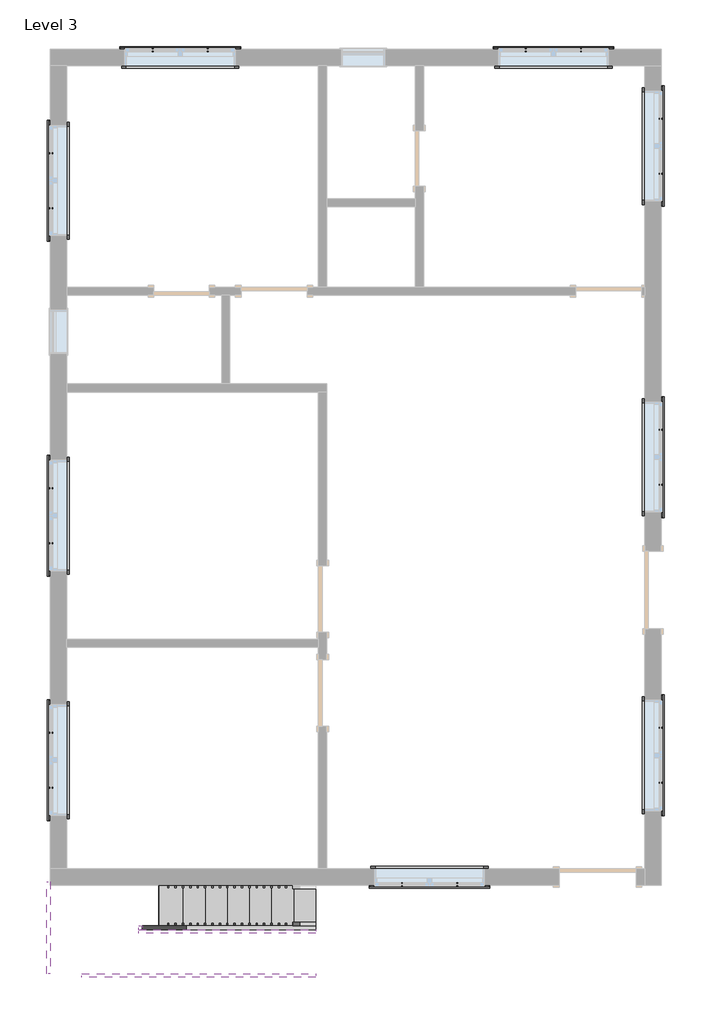
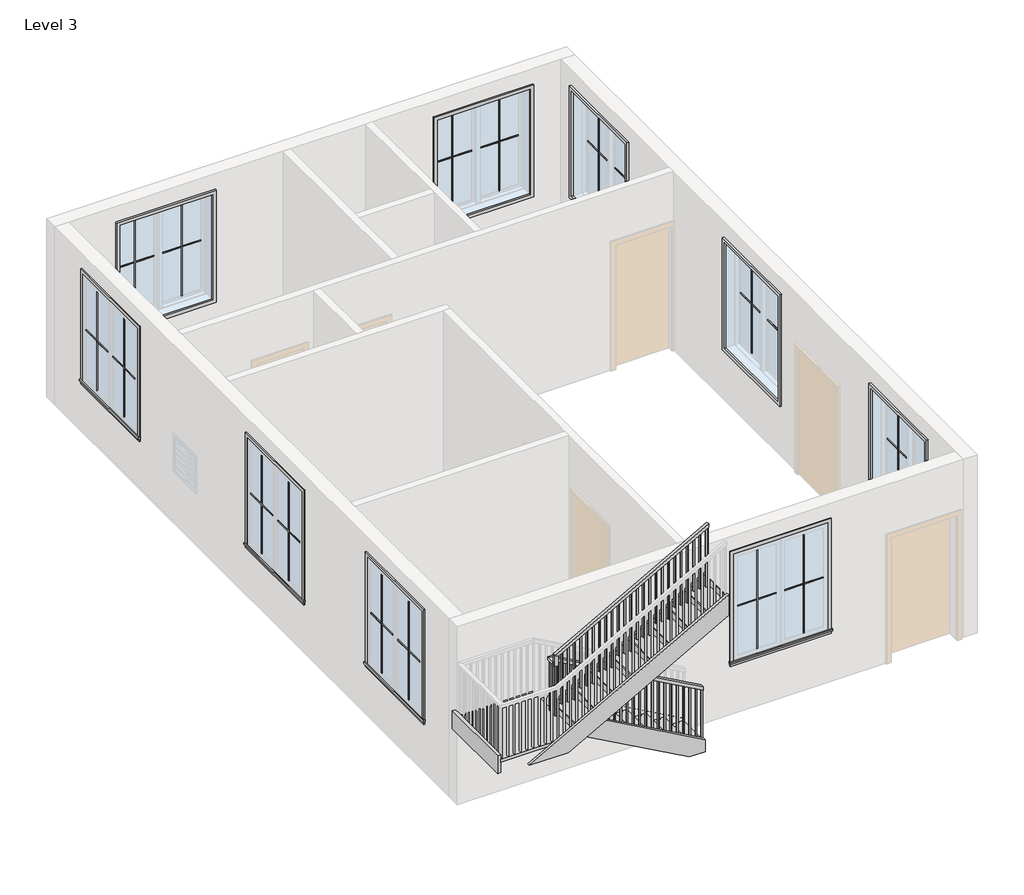
# One storey, part 3 of 3: 36 proxies, 6 members, 1 railing, 1 stair flight.
"""IFC4 building model written with IfcOpenShell, lengths in millimetres."""

from ifc_helpers import new_model, si_unit, frame, origin, place, context, project, spatial, polyline, outline, extrude, faceted_brep, transform, mapped, element, save
from components import muntin_pattern_2x2_muntin_pattern_2x2_f6a80940, muntin_pattern_2x2_muntin_pattern_2x2_09b00a1c, trim_window_exterior_flat_with_sill_698ed857, trim_window_interior_flat_picture_frame_92551a5e, stair_flight_17867b1e

model = new_model("IFC4")

# Units and contexts
model_context = context("Model", 3, world=origin())
ifc_project = project(units=[si_unit("LENGTHUNIT", "METRE", prefix="MILLI")], contexts=[model_context])

# Site, building, storey
site = spatial("IfcSite", under=ifc_project)
building = spatial("IfcBuilding", under=site)
storey = spatial("IfcBuildingStorey", under=building, Name="Level 3", Elevation=3200.4)

# Proxies
placement = place(None, origin())
muntin_pattern_2x2_muntin_pattern_2x2_shape = muntin_pattern_2x2_muntin_pattern_2x2_f6a80940(model_context)
element("IfcBuildingElementProxy", 1, Name="Muntin Pattern_2x2 : Muntin Pattern_2x2", ObjectType="Muntin Pattern_2x2 : Muntin Pattern_2x2", at=placement, inside=storey, context=model_context, shape_type="MappedRepresentation", body=[
    mapped(muntin_pattern_2x2_muntin_pattern_2x2_shape, transform((-5453.9948569, -3961.7808037, 4184.65), x_axis=(0.0, 1.0, 0.0), y_axis=(-1.0, 0.0, 0.0), z_axis=(0.0, 0.0, 1.0))),
])
element("IfcBuildingElementProxy", 2, Name="Muntin Pattern_2x2 : Muntin Pattern_2x2", ObjectType="Muntin Pattern_2x2 : Muntin Pattern_2x2", at=placement, inside=storey, context=model_context, shape_type="MappedRepresentation", body=[
    mapped(muntin_pattern_2x2_muntin_pattern_2x2_shape, transform((-5453.9948569, -593.1058037, 4184.65), x_axis=(0.0, 1.0, 0.0), y_axis=(-1.0, 0.0, 0.0), z_axis=(0.0, 0.0, 1.0))),
])
element("IfcBuildingElementProxy", 3, Name="Muntin Pattern_2x2 : Muntin Pattern_2x2", ObjectType="Muntin Pattern_2x2 : Muntin Pattern_2x2", at=placement, inside=storey, context=model_context, shape_type="MappedRepresentation", body=[
    mapped(muntin_pattern_2x2_muntin_pattern_2x2_shape, transform((-5453.9948569, 4023.3441963, 4184.65), x_axis=(0.0, 1.0, 0.0), y_axis=(-1.0, 0.0, 0.0), z_axis=(0.0, 0.0, 1.0))),
])
element("IfcBuildingElementProxy", 4, Name="Muntin Pattern_2x2 : Muntin Pattern_2x2", ObjectType="Muntin Pattern_2x2 : Muntin Pattern_2x2", at=placement, inside=storey, context=model_context, shape_type="MappedRepresentation", body=[
    mapped(muntin_pattern_2x2_muntin_pattern_2x2_shape, transform((2947.0551431, 5258.4191963, 4184.65), x_axis=(0.0, -1.0, 0.0), y_axis=(1.0, 0.0, 0.0), z_axis=(0.0, 0.0, 1.0))),
])
element("IfcBuildingElementProxy", 5, Name="Muntin Pattern_2x2 : Muntin Pattern_2x2", ObjectType="Muntin Pattern_2x2 : Muntin Pattern_2x2", at=placement, inside=storey, context=model_context, shape_type="MappedRepresentation", body=[
    mapped(muntin_pattern_2x2_muntin_pattern_2x2_shape, transform((2947.0551431, 972.1691963, 4184.65), x_axis=(0.0, -1.0, 0.0), y_axis=(1.0, 0.0, 0.0), z_axis=(0.0, 0.0, 1.0))),
])
element("IfcBuildingElementProxy", 6, Name="Muntin Pattern_2x2 : Muntin Pattern_2x2", ObjectType="Muntin Pattern_2x2 : Muntin Pattern_2x2", at=placement, inside=storey, context=model_context, shape_type="MappedRepresentation", body=[
    mapped(muntin_pattern_2x2_muntin_pattern_2x2_shape, transform((2947.0551431, -3136.2808037, 4184.65), x_axis=(0.0, -1.0, 0.0), y_axis=(1.0, 0.0, 0.0), z_axis=(0.0, 0.0, 1.0))),
])
element("IfcBuildingElementProxy", 7, Name="Muntin Pattern_2x2 : Muntin Pattern_2x2", ObjectType="Muntin Pattern_2x2 : Muntin Pattern_2x2", at=placement, inside=storey, context=model_context, shape_type="MappedRepresentation", body=[
    mapped(muntin_pattern_2x2_muntin_pattern_2x2_shape, transform((141.9426431, -5296.8683037, 4184.65), x_axis=(-1.0, 0.0, 0.0), y_axis=(0.0, -1.0, 0.0), z_axis=(0.0, 0.0, 1.0))),
])
element("IfcBuildingElementProxy", 8, Name="Muntin Pattern_2x2 : Muntin Pattern_2x2", ObjectType="Muntin Pattern_2x2 : Muntin Pattern_2x2", at=placement, inside=storey, context=model_context, shape_type="MappedRepresentation", body=[
    mapped(muntin_pattern_2x2_muntin_pattern_2x2_shape, transform((1091.2676431, 6202.9816963, 4184.65), x_axis=(1.0, 0.0, 0.0), y_axis=(0.0, 1.0, 0.0), z_axis=(0.0, 0.0, 1.0))),
])
element("IfcBuildingElementProxy", 9, Name="Muntin Pattern_2x2 : Muntin Pattern_2x2", ObjectType="Muntin Pattern_2x2 : Muntin Pattern_2x2", at=placement, inside=storey, context=model_context, shape_type="MappedRepresentation", body=[
    mapped(muntin_pattern_2x2_muntin_pattern_2x2_shape, transform((-4052.2323569, 6202.9816963, 4184.65), x_axis=(1.0, 0.0, 0.0), y_axis=(0.0, 1.0, 0.0), z_axis=(0.0, 0.0, 1.0))),
])
muntin_pattern_2x2_muntin_pattern_2x2_2_shape = muntin_pattern_2x2_muntin_pattern_2x2_09b00a1c(model_context)
element("IfcBuildingElementProxy", 10, Name="Muntin Pattern_2x2 : Muntin Pattern_2x2", ObjectType="Muntin Pattern_2x2 : Muntin Pattern_2x2", at=placement, inside=storey, context=model_context, shape_type="MappedRepresentation", body=[
    mapped(muntin_pattern_2x2_muntin_pattern_2x2_2_shape, transform((-5453.9948569, -3202.9558037, 4184.65), x_axis=(0.0, -1.0, 0.0), y_axis=(1.0, 0.0, 0.0), z_axis=(0.0, 0.0, 1.0))),
])
element("IfcBuildingElementProxy", 11, Name="Muntin Pattern_2x2 : Muntin Pattern_2x2", ObjectType="Muntin Pattern_2x2 : Muntin Pattern_2x2", at=placement, inside=storey, context=model_context, shape_type="MappedRepresentation", body=[
    mapped(muntin_pattern_2x2_muntin_pattern_2x2_2_shape, transform((-5453.9948569, 165.7191963, 4184.65), x_axis=(0.0, -1.0, 0.0), y_axis=(1.0, 0.0, 0.0), z_axis=(0.0, 0.0, 1.0))),
])
element("IfcBuildingElementProxy", 12, Name="Muntin Pattern_2x2 : Muntin Pattern_2x2", ObjectType="Muntin Pattern_2x2 : Muntin Pattern_2x2", at=placement, inside=storey, context=model_context, shape_type="MappedRepresentation", body=[
    mapped(muntin_pattern_2x2_muntin_pattern_2x2_2_shape, transform((-5453.9948569, 4782.1691963, 4184.65), x_axis=(0.0, -1.0, 0.0), y_axis=(1.0, 0.0, 0.0), z_axis=(0.0, 0.0, 1.0))),
])
element("IfcBuildingElementProxy", 13, Name="Muntin Pattern_2x2 : Muntin Pattern_2x2", ObjectType="Muntin Pattern_2x2 : Muntin Pattern_2x2", at=placement, inside=storey, context=model_context, shape_type="MappedRepresentation", body=[
    mapped(muntin_pattern_2x2_muntin_pattern_2x2_2_shape, transform((2947.0551431, 4499.5941963, 4184.65), x_axis=(0.0, 1.0, 0.0), y_axis=(-1.0, 0.0, 0.0), z_axis=(0.0, 0.0, 1.0))),
])
element("IfcBuildingElementProxy", 14, Name="Muntin Pattern_2x2 : Muntin Pattern_2x2", ObjectType="Muntin Pattern_2x2 : Muntin Pattern_2x2", at=placement, inside=storey, context=model_context, shape_type="MappedRepresentation", body=[
    mapped(muntin_pattern_2x2_muntin_pattern_2x2_2_shape, transform((2947.0551431, 213.3441963, 4184.65), x_axis=(0.0, 1.0, 0.0), y_axis=(-1.0, 0.0, 0.0), z_axis=(0.0, 0.0, 1.0))),
])
element("IfcBuildingElementProxy", 15, Name="Muntin Pattern_2x2 : Muntin Pattern_2x2", ObjectType="Muntin Pattern_2x2 : Muntin Pattern_2x2", at=placement, inside=storey, context=model_context, shape_type="MappedRepresentation", body=[
    mapped(muntin_pattern_2x2_muntin_pattern_2x2_2_shape, transform((2947.0551431, -3895.1058037, 4184.65), x_axis=(0.0, 1.0, 0.0), y_axis=(-1.0, 0.0, 0.0), z_axis=(0.0, 0.0, 1.0))),
])
element("IfcBuildingElementProxy", 16, Name="Muntin Pattern_2x2 : Muntin Pattern_2x2", ObjectType="Muntin Pattern_2x2 : Muntin Pattern_2x2", at=placement, inside=storey, context=model_context, shape_type="MappedRepresentation", body=[
    mapped(muntin_pattern_2x2_muntin_pattern_2x2_2_shape, transform((-616.8823569, -5296.8683037, 4184.65), x_axis=(1.0, 0.0, 0.0), y_axis=(0.0, 1.0, 0.0), z_axis=(0.0, 0.0, 1.0))),
])
element("IfcBuildingElementProxy", 17, Name="Muntin Pattern_2x2 : Muntin Pattern_2x2", ObjectType="Muntin Pattern_2x2 : Muntin Pattern_2x2", at=placement, inside=storey, context=model_context, shape_type="MappedRepresentation", body=[
    mapped(muntin_pattern_2x2_muntin_pattern_2x2_2_shape, transform((1850.0926431, 6202.9816963, 4184.65), x_axis=(-1.0, 0.0, 0.0), y_axis=(0.0, -1.0, 0.0), z_axis=(0.0, 0.0, 1.0))),
])
element("IfcBuildingElementProxy", 18, Name="Muntin Pattern_2x2 : Muntin Pattern_2x2", ObjectType="Muntin Pattern_2x2 : Muntin Pattern_2x2", at=placement, inside=storey, context=model_context, shape_type="MappedRepresentation", body=[
    mapped(muntin_pattern_2x2_muntin_pattern_2x2_2_shape, transform((-3293.4073569, 6202.9816963, 4184.65), x_axis=(-1.0, 0.0, 0.0), y_axis=(0.0, -1.0, 0.0), z_axis=(0.0, 0.0, 1.0))),
])
trim_window_exterior_flat_with_sill_shape = trim_window_exterior_flat_with_sill_698ed857(model_context)
element("IfcBuildingElementProxy", 19, Name="Trim-Window-Exterior-Flat : with Sill", ObjectType="Trim-Window-Exterior-Flat : with Sill", at=placement, inside=storey, context=model_context, shape_type="MappedRepresentation", body=[
    mapped(trim_window_exterior_flat_with_sill_shape, transform((-5463.5198569, -3582.3683037, 5943.6), x_axis=(0.0, -1.0, 0.0), y_axis=(0.0, 0.0, 1.0), z_axis=(-1.0, 0.0, 0.0))),
])
element("IfcBuildingElementProxy", 20, Name="Trim-Window-Exterior-Flat : with Sill", ObjectType="Trim-Window-Exterior-Flat : with Sill", at=placement, inside=storey, context=model_context, shape_type="MappedRepresentation", body=[
    mapped(trim_window_exterior_flat_with_sill_shape, transform((-5463.5198569, -213.6933037, 5943.6), x_axis=(0.0, -1.0, 0.0), y_axis=(0.0, 0.0, 1.0), z_axis=(-1.0, 0.0, 0.0))),
])
element("IfcBuildingElementProxy", 21, Name="Trim-Window-Exterior-Flat : with Sill", ObjectType="Trim-Window-Exterior-Flat : with Sill", at=placement, inside=storey, context=model_context, shape_type="MappedRepresentation", body=[
    mapped(trim_window_exterior_flat_with_sill_shape, transform((-5463.5198569, 4402.7566963, 5943.6), x_axis=(0.0, -1.0, 0.0), y_axis=(0.0, 0.0, 1.0), z_axis=(-1.0, 0.0, 0.0))),
])
element("IfcBuildingElementProxy", 22, Name="Trim-Window-Exterior-Flat : with Sill", ObjectType="Trim-Window-Exterior-Flat : with Sill", at=placement, inside=storey, context=model_context, shape_type="MappedRepresentation", body=[
    mapped(trim_window_exterior_flat_with_sill_shape, transform((2956.5801431, 4879.0066963, 5943.6), x_axis=(0.0, 1.0, 0.0), y_axis=(0.0, 0.0, 1.0), z_axis=(1.0, 0.0, 0.0))),
])
element("IfcBuildingElementProxy", 23, Name="Trim-Window-Exterior-Flat : with Sill", ObjectType="Trim-Window-Exterior-Flat : with Sill", at=placement, inside=storey, context=model_context, shape_type="MappedRepresentation", body=[
    mapped(trim_window_exterior_flat_with_sill_shape, transform((2956.5801431, 592.7566963, 5943.6), x_axis=(0.0, 1.0, 0.0), y_axis=(0.0, 0.0, 1.0), z_axis=(1.0, 0.0, 0.0))),
])
element("IfcBuildingElementProxy", 24, Name="Trim-Window-Exterior-Flat : with Sill", ObjectType="Trim-Window-Exterior-Flat : with Sill", at=placement, inside=storey, context=model_context, shape_type="MappedRepresentation", body=[
    mapped(trim_window_exterior_flat_with_sill_shape, transform((2956.5801431, -3515.6933037, 5943.6), x_axis=(0.0, 1.0, 0.0), y_axis=(0.0, 0.0, 1.0), z_axis=(1.0, 0.0, 0.0))),
])
element("IfcBuildingElementProxy", 25, Name="Trim-Window-Exterior-Flat : with Sill", ObjectType="Trim-Window-Exterior-Flat : with Sill", at=placement, inside=storey, context=model_context, shape_type="MappedRepresentation", body=[
    mapped(trim_window_exterior_flat_with_sill_shape, transform((-237.4698569, -5306.3933037, 5943.6), x_axis=(1.0, 0.0, 0.0), y_axis=(0.0, 0.0, 1.0), z_axis=(0.0, -1.0, 0.0))),
])
element("IfcBuildingElementProxy", 26, Name="Trim-Window-Exterior-Flat : with Sill", ObjectType="Trim-Window-Exterior-Flat : with Sill", at=placement, inside=storey, context=model_context, shape_type="MappedRepresentation", body=[
    mapped(trim_window_exterior_flat_with_sill_shape, transform((1470.6801431, 6212.5066963, 5943.6), x_axis=(-1.0, 0.0, 0.0), y_axis=(0.0, 0.0, 1.0), z_axis=(0.0, 1.0, 0.0))),
])
element("IfcBuildingElementProxy", 27, Name="Trim-Window-Exterior-Flat : with Sill", ObjectType="Trim-Window-Exterior-Flat : with Sill", at=placement, inside=storey, context=model_context, shape_type="MappedRepresentation", body=[
    mapped(trim_window_exterior_flat_with_sill_shape, transform((-3672.8198569, 6212.5066963, 5943.6), x_axis=(-1.0, 0.0, 0.0), y_axis=(0.0, 0.0, 1.0), z_axis=(0.0, 1.0, 0.0))),
])
trim_window_interior_flat_picture_frame_shape = trim_window_interior_flat_picture_frame_92551a5e(model_context)
element("IfcBuildingElementProxy", 28, Name="Trim-Window-Interior-Flat : Picture Frame", ObjectType="Trim-Window-Interior-Flat : Picture Frame", at=placement, inside=storey, context=model_context, shape_type="MappedRepresentation", body=[
    mapped(trim_window_interior_flat_picture_frame_shape, transform((-5234.9198569, -3582.3683037, 5943.6), x_axis=(0.0, 1.0, 0.0), y_axis=(0.0, 0.0, 1.0), z_axis=(1.0, 0.0, 0.0))),
])
element("IfcBuildingElementProxy", 29, Name="Trim-Window-Interior-Flat : Picture Frame", ObjectType="Trim-Window-Interior-Flat : Picture Frame", at=placement, inside=storey, context=model_context, shape_type="MappedRepresentation", body=[
    mapped(trim_window_interior_flat_picture_frame_shape, transform((-5234.9198569, -213.6933037, 5943.6), x_axis=(0.0, 1.0, 0.0), y_axis=(0.0, 0.0, 1.0), z_axis=(1.0, 0.0, 0.0))),
])
element("IfcBuildingElementProxy", 30, Name="Trim-Window-Interior-Flat : Picture Frame", ObjectType="Trim-Window-Interior-Flat : Picture Frame", at=placement, inside=storey, context=model_context, shape_type="MappedRepresentation", body=[
    mapped(trim_window_interior_flat_picture_frame_shape, transform((-5234.9198569, 4402.7566963, 5943.6), x_axis=(0.0, 1.0, 0.0), y_axis=(0.0, 0.0, 1.0), z_axis=(1.0, 0.0, 0.0))),
])
element("IfcBuildingElementProxy", 31, Name="Trim-Window-Interior-Flat : Picture Frame", ObjectType="Trim-Window-Interior-Flat : Picture Frame", at=placement, inside=storey, context=model_context, shape_type="MappedRepresentation", body=[
    mapped(trim_window_interior_flat_picture_frame_shape, transform((2727.9801431, 4879.0066963, 5943.6), x_axis=(0.0, -1.0, 0.0), y_axis=(0.0, 0.0, 1.0), z_axis=(-1.0, 0.0, 0.0))),
])
element("IfcBuildingElementProxy", 32, Name="Trim-Window-Interior-Flat : Picture Frame", ObjectType="Trim-Window-Interior-Flat : Picture Frame", at=placement, inside=storey, context=model_context, shape_type="MappedRepresentation", body=[
    mapped(trim_window_interior_flat_picture_frame_shape, transform((2727.9801431, 592.7566963, 5943.6), x_axis=(0.0, -1.0, 0.0), y_axis=(0.0, 0.0, 1.0), z_axis=(-1.0, 0.0, 0.0))),
])
element("IfcBuildingElementProxy", 33, Name="Trim-Window-Interior-Flat : Picture Frame", ObjectType="Trim-Window-Interior-Flat : Picture Frame", at=placement, inside=storey, context=model_context, shape_type="MappedRepresentation", body=[
    mapped(trim_window_interior_flat_picture_frame_shape, transform((2727.9801431, -3515.6933037, 5943.6), x_axis=(0.0, -1.0, 0.0), y_axis=(0.0, 0.0, 1.0), z_axis=(-1.0, 0.0, 0.0))),
])
element("IfcBuildingElementProxy", 34, Name="Trim-Window-Interior-Flat : Picture Frame", ObjectType="Trim-Window-Interior-Flat : Picture Frame", at=placement, inside=storey, context=model_context, shape_type="MappedRepresentation", body=[
    mapped(trim_window_interior_flat_picture_frame_shape, transform((-237.4698569, -5077.7933037, 5943.6), x_axis=(-1.0, 0.0, 0.0), y_axis=(0.0, 0.0, 1.0), z_axis=(0.0, 1.0, 0.0))),
])
element("IfcBuildingElementProxy", 35, Name="Trim-Window-Interior-Flat : Picture Frame", ObjectType="Trim-Window-Interior-Flat : Picture Frame", at=placement, inside=storey, context=model_context, shape_type="MappedRepresentation", body=[
    mapped(trim_window_interior_flat_picture_frame_shape, transform((1470.6801431, 5983.9066963, 5943.6), x_axis=(1.0, 0.0, 0.0), y_axis=(0.0, 0.0, 1.0), z_axis=(0.0, -1.0, 0.0))),
])
element("IfcBuildingElementProxy", 36, Name="Trim-Window-Interior-Flat : Picture Frame", ObjectType="Trim-Window-Interior-Flat : Picture Frame", at=placement, inside=storey, context=model_context, shape_type="MappedRepresentation", body=[
    mapped(trim_window_interior_flat_picture_frame_shape, transform((-3672.8198569, 5983.9066963, 5943.6), x_axis=(1.0, 0.0, 0.0), y_axis=(0.0, 0.0, 1.0), z_axis=(0.0, -1.0, 0.0))),
])

# Members
element("IfcMember", 37, ObjectType="Stringer - 2\" Width", at=placement, inside=storey, context=model_context, shape_type="SweptSolid", body=[
    extrude(outline(polyline([(3200.4, -1805.9198569), (3407.9983948, -1805.9198569), (4734.4428392, -4193.5198569), (4385.7641651, -4193.5198569), (3200.4, -2059.8643597), (3200.4, -1805.9198569)])), frame((0.0, -5915.9933037, 0.0), z_axis=(0.0, 1.0, 0.0), x_axis=(0.0, 0.0, 1.0)), (0.0, 0.0, 1.0), 50.8),
])
element("IfcMember", 38, ObjectType="Stringer - 2\" Width", at=placement, inside=storey, context=model_context, shape_type="SweptSolid", body=[
    extrude(outline(polyline([(-4244.3198569, -5865.1933037), (-4193.5198569, -5865.1933037), (-4193.5198569, -5915.9933037), (-4244.3198569, -5915.9933037), (-4244.3198569, -5865.1933037)])), frame((0.0, 0.0, 4495.8), z_axis=(0.0, 0.0, 1.0), x_axis=(1.0, 0.0, 0.0)), (0.0, 0.0, 1.0), 304.8),
])
element("IfcMember", 39, ObjectType="Stringer - 2\" Width", at=placement, inside=storey, context=model_context, shape_type="SweptSolid", body=[
    extrude(outline(polyline([(4931.9983948, -4244.3198569), (4583.3197207, -4244.3198569), (5937.9863873, -1805.9198569), (6286.6650614, -1805.9198569), (4931.9983948, -4244.3198569)])), frame((0.0, -5966.7933037, 0.0), z_axis=(0.0, 1.0, 0.0), x_axis=(0.0, 0.0, 1.0)), (0.0, 0.0, 1.0), 50.8),
])
element("IfcMember", 40, ObjectType="Stringer - 2\" Width", at=placement, inside=storey, context=model_context, shape_type="SweptSolid", body=[
    extrude(outline(polyline([(3200.4, -1805.9198569), (3407.9983948, -1805.9198569), (4800.6, -4312.6027463), (4800.6, -4940.2243597), (3200.4, -2059.8643597), (3200.4, -1805.9198569)])), frame((0.0, -5306.3933037, 0.0), z_axis=(0.0, 1.0, 0.0), x_axis=(0.0, 0.0, 1.0)), (0.0, 0.0, 1.0), 50.8),
])
element("IfcMember", 41, ObjectType="Stringer - 2\" Width", at=placement, inside=storey, context=model_context, shape_type="SweptSolid", body=[
    extrude(outline(polyline([(-5514.3198569, -5255.5933037), (-5463.5198569, -5255.5933037), (-5463.5198569, -6525.5933037), (-5514.3198569, -6525.5933037), (-5514.3198569, -5255.5933037)])), frame((0.0, 0.0, 4495.8), z_axis=(0.0, 0.0, 1.0), x_axis=(1.0, 0.0, 0.0)), (0.0, 0.0, 1.0), 304.8),
])
element("IfcMember", 42, ObjectType="Stringer - 2\" Width", at=placement, inside=storey, context=model_context, shape_type="SweptSolid", body=[
    extrude(outline(polyline([(4495.8, -4401.8553541), (5937.9863873, -1805.9198569), (6286.6650614, -1805.9198569), (4495.8, -5029.4769675), (4495.8, -4401.8553541)])), frame((0.0, -6576.3933037, 0.0), z_axis=(0.0, 1.0, 0.0), x_axis=(0.0, 0.0, 1.0)), (0.0, 0.0, 1.0), 50.8),
])

# Railing
element("IfcRailing", 43, ObjectType="Handrail - Rectangular", at=placement, inside=storey, context=model_context, shape_type="SolidModel", body=[
    faceted_brep([(-1805.9198569, -5865.1933037, 4284.1333333), (-1805.9198569, -5865.1933037, 4226.020221), (-1805.9198569, -5814.3933037, 4226.020221), (-1805.9198569, -5814.3933037, 4284.1333333), (-4168.1198569, -5865.1933037, 5596.4666667), (-4218.9198569, -5865.1933037, 5566.5757765), (-4218.9198569, -5814.3933037, 5566.5757765), (-4168.1198569, -5814.3933037, 5596.4666667), (-4168.1198569, -5865.1933037, 5638.8), (-4218.9198569, -5865.1933037, 5588.0), (-4218.9198569, -5814.3933037, 5588.0), (-4168.1198569, -5814.3933037, 5638.8), (-4244.3198569, -5865.1933037, 5638.8), (-4244.3198569, -5865.1933037, 5588.0), (-4295.1198569, -5814.3933037, 5588.0), (-4295.1198569, -5814.3933037, 5638.8), (-4244.3198569, -5941.3933037, 5638.8), (-4244.3198569, -5941.3933037, 5588.0), (-4295.1198569, -5941.3933037, 5588.0), (-4295.1198569, -5941.3933037, 5638.8), (-4244.3198569, -5966.7933037, 5638.8), (-4295.1198569, -5966.7933037, 5638.8), (-4295.1198569, -6017.5933037, 5588.0), (-4244.3198569, -6017.5933037, 5588.0)], [[[0, 1, 2, 3]], [[1, 0, 4, 5]], [[2, 1, 5, 6]], [[3, 2, 6, 7]], [[0, 3, 7, 4]], [[5, 4, 8, 9]], [[6, 5, 9, 10]], [[7, 6, 10, 11]], [[4, 7, 11, 8]], [[9, 8, 12, 13]], [[10, 9, 13, 14]], [[11, 10, 14, 15]], [[8, 11, 15, 12]], [[13, 12, 16, 17]], [[14, 13, 17, 18]], [[15, 14, 18, 19]], [[12, 15, 19, 16]], [[20, 21, 22, 23]], [[17, 16, 20, 23]], [[18, 17, 23, 22]], [[19, 18, 22, 21]], [[16, 19, 21, 20]]]),
    faceted_brep([(-4244.3198569, -5966.7933037, 5638.8), (-4244.3198569, -6017.5933037, 5588.0), (-4295.1198569, -6017.5933037, 5588.0), (-4295.1198569, -5966.7933037, 5638.8), (-4244.3198569, -5966.7933037, 5750.020221), (-4295.1198569, -5966.7933037, 5779.9111111), (-4295.1198569, -6017.5933037, 5779.9111111), (-4244.3198569, -6017.5933037, 5750.020221)], [[[0, 1, 2, 3]], [[4, 5, 6, 7]], [[1, 0, 4, 7]], [[2, 1, 7, 6]], [[3, 2, 6, 5]], [[0, 3, 5, 4]]]),
    faceted_brep([(-4295.1198569, -5966.7933037, 5779.9111111), (-4244.3198569, -5966.7933037, 5750.020221), (-4244.3198569, -6017.5933037, 5750.020221), (-4295.1198569, -6017.5933037, 5779.9111111), (-1805.9198569, -5966.7933037, 7162.8), (-1805.9198569, -6017.5933037, 7162.8), (-1805.9198569, -6017.5933037, 7104.6868876), (-1805.9198569, -5966.7933037, 7104.6868876)], [[[0, 1, 2, 3]], [[4, 5, 6, 7]], [[1, 0, 4, 7]], [[2, 1, 7, 6]], [[3, 2, 6, 5]], [[0, 3, 5, 4]]]),
    extrude(outline(polyline([(7085.2841099, -1840.8448569), (6079.0666667, -1840.8448569), (6079.0666667, -1821.7948569), (7095.8674432, -1821.7948569), (7085.2841099, -1840.8448569)])), frame((0.0, -6001.7183037, 0.0), z_axis=(0.0, 1.0, 0.0), x_axis=(0.0, 0.0, 1.0)), (0.0, 0.0, 1.0), 19.05),
    extrude(outline(polyline([(7028.8396654, -1942.4448569), (6079.0666667, -1942.4448569), (6079.0666667, -1923.3948569), (7039.4229988, -1923.3948569), (7028.8396654, -1942.4448569)])), frame((0.0, -6001.7183037, 0.0), z_axis=(0.0, 1.0, 0.0), x_axis=(0.0, 0.0, 1.0)), (0.0, 0.0, 1.0), 19.05),
    extrude(outline(polyline([(6972.395221, -2044.0448569), (6079.0666667, -2044.0448569), (6079.0666667, -2024.9948569), (6982.9785543, -2024.9948569), (6972.395221, -2044.0448569)])), frame((0.0, -6001.7183037, 0.0), z_axis=(0.0, 1.0, 0.0), x_axis=(0.0, 0.0, 1.0)), (0.0, 0.0, 1.0), 19.05),
    extrude(outline(polyline([(6915.9507765, -2145.6448569), (5909.7333333, -2145.6448569), (5909.7333333, -2126.5948569), (6926.5341099, -2126.5948569), (6915.9507765, -2145.6448569)])), frame((0.0, -6001.7183037, 0.0), z_axis=(0.0, 1.0, 0.0), x_axis=(0.0, 0.0, 1.0)), (0.0, 0.0, 1.0), 19.05),
    extrude(outline(polyline([(6859.5063321, -2247.2448569), (5909.7333333, -2247.2448569), (5909.7333333, -2228.1948569), (6870.0896654, -2228.1948569), (6859.5063321, -2247.2448569)])), frame((0.0, -6001.7183037, 0.0), z_axis=(0.0, 1.0, 0.0), x_axis=(0.0, 0.0, 1.0)), (0.0, 0.0, 1.0), 19.05),
    extrude(outline(polyline([(6803.0618876, -2348.8448569), (5909.7333333, -2348.8448569), (5909.7333333, -2329.7948569), (6813.645221, -2329.7948569), (6803.0618876, -2348.8448569)])), frame((0.0, -6001.7183037, 0.0), z_axis=(0.0, 1.0, 0.0), x_axis=(0.0, 0.0, 1.0)), (0.0, 0.0, 1.0), 19.05),
    extrude(outline(polyline([(6746.6174432, -2450.4448569), (5740.4, -2450.4448569), (5740.4, -2431.3948569), (6757.2007765, -2431.3948569), (6746.6174432, -2450.4448569)])), frame((0.0, -6001.7183037, 0.0), z_axis=(0.0, 1.0, 0.0), x_axis=(0.0, 0.0, 1.0)), (0.0, 0.0, 1.0), 19.05),
    extrude(outline(polyline([(6690.1729988, -2552.0448569), (5740.4, -2552.0448569), (5740.4, -2532.9948569), (6700.7563321, -2532.9948569), (6690.1729988, -2552.0448569)])), frame((0.0, -6001.7183037, 0.0), z_axis=(0.0, 1.0, 0.0), x_axis=(0.0, 0.0, 1.0)), (0.0, 0.0, 1.0), 19.05),
    extrude(outline(polyline([(6633.7285543, -2653.6448569), (5740.4, -2653.6448569), (5740.4, -2634.5948569), (6644.3118876, -2634.5948569), (6633.7285543, -2653.6448569)])), frame((0.0, -6001.7183037, 0.0), z_axis=(0.0, 1.0, 0.0), x_axis=(0.0, 0.0, 1.0)), (0.0, 0.0, 1.0), 19.05),
    extrude(outline(polyline([(6577.2841099, -2755.2448569), (5571.0666667, -2755.2448569), (5571.0666667, -2736.1948569), (6587.8674432, -2736.1948569), (6577.2841099, -2755.2448569)])), frame((0.0, -6001.7183037, 0.0), z_axis=(0.0, 1.0, 0.0), x_axis=(0.0, 0.0, 1.0)), (0.0, 0.0, 1.0), 19.05),
    extrude(outline(polyline([(6520.8396654, -2856.8448569), (5571.0666667, -2856.8448569), (5571.0666667, -2837.7948569), (6531.4229988, -2837.7948569), (6520.8396654, -2856.8448569)])), frame((0.0, -6001.7183037, 0.0), z_axis=(0.0, 1.0, 0.0), x_axis=(0.0, 0.0, 1.0)), (0.0, 0.0, 1.0), 19.05),
    extrude(outline(polyline([(6464.395221, -2958.4448569), (5571.0666667, -2958.4448569), (5571.0666667, -2939.3948569), (6474.9785543, -2939.3948569), (6464.395221, -2958.4448569)])), frame((0.0, -6001.7183037, 0.0), z_axis=(0.0, 1.0, 0.0), x_axis=(0.0, 0.0, 1.0)), (0.0, 0.0, 1.0), 19.05),
    extrude(outline(polyline([(6407.9507765, -3060.0448569), (5401.7333333, -3060.0448569), (5401.7333333, -3040.9948569), (6418.5341099, -3040.9948569), (6407.9507765, -3060.0448569)])), frame((0.0, -6001.7183037, 0.0), z_axis=(0.0, 1.0, 0.0), x_axis=(0.0, 0.0, 1.0)), (0.0, 0.0, 1.0), 19.05),
    extrude(outline(polyline([(6351.5063321, -3161.6448569), (5401.7333333, -3161.6448569), (5401.7333333, -3142.5948569), (6362.0896654, -3142.5948569), (6351.5063321, -3161.6448569)])), frame((0.0, -6001.7183037, 0.0), z_axis=(0.0, 1.0, 0.0), x_axis=(0.0, 0.0, 1.0)), (0.0, 0.0, 1.0), 19.05),
    extrude(outline(polyline([(6295.0618876, -3263.2448569), (5401.7333333, -3263.2448569), (5401.7333333, -3244.1948569), (6305.645221, -3244.1948569), (6295.0618876, -3263.2448569)])), frame((0.0, -6001.7183037, 0.0), z_axis=(0.0, 1.0, 0.0), x_axis=(0.0, 0.0, 1.0)), (0.0, 0.0, 1.0), 19.05),
    extrude(outline(polyline([(6238.6174432, -3364.8448569), (5232.4, -3364.8448569), (5232.4, -3345.7948569), (6249.2007765, -3345.7948569), (6238.6174432, -3364.8448569)])), frame((0.0, -6001.7183037, 0.0), z_axis=(0.0, 1.0, 0.0), x_axis=(0.0, 0.0, 1.0)), (0.0, 0.0, 1.0), 19.05),
    extrude(outline(polyline([(6182.1729988, -3466.4448569), (5232.4, -3466.4448569), (5232.4, -3447.3948569), (6192.7563321, -3447.3948569), (6182.1729988, -3466.4448569)])), frame((0.0, -6001.7183037, 0.0), z_axis=(0.0, 1.0, 0.0), x_axis=(0.0, 0.0, 1.0)), (0.0, 0.0, 1.0), 19.05),
    extrude(outline(polyline([(6125.7285543, -3568.0448569), (5232.4, -3568.0448569), (5232.4, -3548.9948569), (6136.3118876, -3548.9948569), (6125.7285543, -3568.0448569)])), frame((0.0, -6001.7183037, 0.0), z_axis=(0.0, 1.0, 0.0), x_axis=(0.0, 0.0, 1.0)), (0.0, 0.0, 1.0), 19.05),
    extrude(outline(polyline([(6069.2841099, -3669.6448569), (5063.0666667, -3669.6448569), (5063.0666667, -3650.5948569), (6079.8674432, -3650.5948569), (6069.2841099, -3669.6448569)])), frame((0.0, -6001.7183037, 0.0), z_axis=(0.0, 1.0, 0.0), x_axis=(0.0, 0.0, 1.0)), (0.0, 0.0, 1.0), 19.05),
    extrude(outline(polyline([(6012.8396654, -3771.2448569), (5063.0666667, -3771.2448569), (5063.0666667, -3752.1948569), (6023.4229988, -3752.1948569), (6012.8396654, -3771.2448569)])), frame((0.0, -6001.7183037, 0.0), z_axis=(0.0, 1.0, 0.0), x_axis=(0.0, 0.0, 1.0)), (0.0, 0.0, 1.0), 19.05),
    extrude(outline(polyline([(5956.395221, -3872.8448569), (5063.0666667, -3872.8448569), (5063.0666667, -3853.7948569), (5966.9785543, -3853.7948569), (5956.395221, -3872.8448569)])), frame((0.0, -6001.7183037, 0.0), z_axis=(0.0, 1.0, 0.0), x_axis=(0.0, 0.0, 1.0)), (0.0, 0.0, 1.0), 19.05),
    extrude(outline(polyline([(5899.9507765, -3974.4448569), (4893.7333333, -3974.4448569), (4893.7333333, -3955.3948569), (5910.5341099, -3955.3948569), (5899.9507765, -3974.4448569)])), frame((0.0, -6001.7183037, 0.0), z_axis=(0.0, 1.0, 0.0), x_axis=(0.0, 0.0, 1.0)), (0.0, 0.0, 1.0), 19.05),
    extrude(outline(polyline([(5843.5063321, -4076.0448569), (4893.7333333, -4076.0448569), (4893.7333333, -4056.9948569), (5854.0896654, -4056.9948569), (5843.5063321, -4076.0448569)])), frame((0.0, -6001.7183037, 0.0), z_axis=(0.0, 1.0, 0.0), x_axis=(0.0, 0.0, 1.0)), (0.0, 0.0, 1.0), 19.05),
    extrude(outline(polyline([(5787.0618876, -4177.6448569), (4893.7333333, -4177.6448569), (4893.7333333, -4158.5948569), (5797.645221, -4158.5948569), (5787.0618876, -4177.6448569)])), frame((0.0, -6001.7183037, 0.0), z_axis=(0.0, 1.0, 0.0), x_axis=(0.0, 0.0, 1.0)), (0.0, 0.0, 1.0), 19.05),
    extrude(outline(polyline([(-4260.1948569, -5931.8683037), (-4260.1948569, -5950.9183037), (-4279.2448569, -5950.9183037), (-4279.2448569, -5931.8683037), (-4260.1948569, -5931.8683037)])), frame((0.0, 0.0, 4724.4), z_axis=(0.0, 0.0, 1.0), x_axis=(1.0, 0.0, 0.0)), (0.0, 0.0, 1.0), 863.6),
    extrude(outline(polyline([(-4234.7948569, -5849.3183037), (-4253.8448569, -5849.3183037), (-4253.8448569, -5830.2683037), (-4234.7948569, -5830.2683037), (-4234.7948569, -5849.3183037)])), frame((0.0, 0.0, 4724.4), z_axis=(0.0, 0.0, 1.0), x_axis=(1.0, 0.0, 0.0)), (0.0, 0.0, 1.0), 863.6),
    extrude(outline(polyline([(5529.5341099, -4152.2448569), (4555.0666667, -4152.2448569), (4555.0666667, -4133.1948569), (5518.9507765, -4133.1948569), (5529.5341099, -4152.2448569)])), frame((0.0, -5849.3183037, 0.0), z_axis=(0.0, 1.0, 0.0), x_axis=(0.0, 0.0, 1.0)), (0.0, 0.0, 1.0), 19.05),
    extrude(outline(polyline([(5473.0896654, -4050.6448569), (4555.0666667, -4050.6448569), (4555.0666667, -4031.5948569), (5462.5063321, -4031.5948569), (5473.0896654, -4050.6448569)])), frame((0.0, -5849.3183037, 0.0), z_axis=(0.0, 1.0, 0.0), x_axis=(0.0, 0.0, 1.0)), (0.0, 0.0, 1.0), 19.05),
    extrude(outline(polyline([(5416.645221, -3949.0448569), (4555.0666667, -3949.0448569), (4555.0666667, -3929.9948569), (5406.0618876, -3929.9948569), (5416.645221, -3949.0448569)])), frame((0.0, -5849.3183037, 0.0), z_axis=(0.0, 1.0, 0.0), x_axis=(0.0, 0.0, 1.0)), (0.0, 0.0, 1.0), 19.05),
    extrude(outline(polyline([(5360.2007765, -3847.4448569), (4385.7333333, -3847.4448569), (4385.7333333, -3828.3948569), (5349.6174432, -3828.3948569), (5360.2007765, -3847.4448569)])), frame((0.0, -5849.3183037, 0.0), z_axis=(0.0, 1.0, 0.0), x_axis=(0.0, 0.0, 1.0)), (0.0, 0.0, 1.0), 19.05),
    extrude(outline(polyline([(5303.7563321, -3745.8448569), (4385.7333333, -3745.8448569), (4385.7333333, -3726.7948569), (5293.1729988, -3726.7948569), (5303.7563321, -3745.8448569)])), frame((0.0, -5849.3183037, 0.0), z_axis=(0.0, 1.0, 0.0), x_axis=(0.0, 0.0, 1.0)), (0.0, 0.0, 1.0), 19.05),
    extrude(outline(polyline([(5247.3118876, -3644.2448569), (4385.7333333, -3644.2448569), (4385.7333333, -3625.1948569), (5236.7285543, -3625.1948569), (5247.3118876, -3644.2448569)])), frame((0.0, -5849.3183037, 0.0), z_axis=(0.0, 1.0, 0.0), x_axis=(0.0, 0.0, 1.0)), (0.0, 0.0, 1.0), 19.05),
    extrude(outline(polyline([(5190.8674432, -3542.6448569), (4216.4, -3542.6448569), (4216.4, -3523.5948569), (5180.2841099, -3523.5948569), (5190.8674432, -3542.6448569)])), frame((0.0, -5849.3183037, 0.0), z_axis=(0.0, 1.0, 0.0), x_axis=(0.0, 0.0, 1.0)), (0.0, 0.0, 1.0), 19.05),
    extrude(outline(polyline([(5134.4229988, -3441.0448569), (4216.4, -3441.0448569), (4216.4, -3421.9948569), (5123.8396654, -3421.9948569), (5134.4229988, -3441.0448569)])), frame((0.0, -5849.3183037, 0.0), z_axis=(0.0, 1.0, 0.0), x_axis=(0.0, 0.0, 1.0)), (0.0, 0.0, 1.0), 19.05),
    extrude(outline(polyline([(5077.9785543, -3339.4448569), (4216.4, -3339.4448569), (4216.4, -3320.3948569), (5067.395221, -3320.3948569), (5077.9785543, -3339.4448569)])), frame((0.0, -5849.3183037, 0.0), z_axis=(0.0, 1.0, 0.0), x_axis=(0.0, 0.0, 1.0)), (0.0, 0.0, 1.0), 19.05),
    extrude(outline(polyline([(5021.5341099, -3237.8448569), (4047.0666667, -3237.8448569), (4047.0666667, -3218.7948569), (5010.9507765, -3218.7948569), (5021.5341099, -3237.8448569)])), frame((0.0, -5849.3183037, 0.0), z_axis=(0.0, 1.0, 0.0), x_axis=(0.0, 0.0, 1.0)), (0.0, 0.0, 1.0), 19.05),
    extrude(outline(polyline([(4965.0896654, -3136.2448569), (4047.0666667, -3136.2448569), (4047.0666667, -3117.1948569), (4954.5063321, -3117.1948569), (4965.0896654, -3136.2448569)])), frame((0.0, -5849.3183037, 0.0), z_axis=(0.0, 1.0, 0.0), x_axis=(0.0, 0.0, 1.0)), (0.0, 0.0, 1.0), 19.05),
    extrude(outline(polyline([(4908.645221, -3034.6448569), (4047.0666667, -3034.6448569), (4047.0666667, -3015.5948569), (4898.0618876, -3015.5948569), (4908.645221, -3034.6448569)])), frame((0.0, -5849.3183037, 0.0), z_axis=(0.0, 1.0, 0.0), x_axis=(0.0, 0.0, 1.0)), (0.0, 0.0, 1.0), 19.05),
    extrude(outline(polyline([(4852.2007765, -2933.0448569), (3877.7333333, -2933.0448569), (3877.7333333, -2913.9948569), (4841.6174432, -2913.9948569), (4852.2007765, -2933.0448569)])), frame((0.0, -5849.3183037, 0.0), z_axis=(0.0, 1.0, 0.0), x_axis=(0.0, 0.0, 1.0)), (0.0, 0.0, 1.0), 19.05),
    extrude(outline(polyline([(4795.7563321, -2831.4448569), (3877.7333333, -2831.4448569), (3877.7333333, -2812.3948569), (4785.1729988, -2812.3948569), (4795.7563321, -2831.4448569)])), frame((0.0, -5849.3183037, 0.0), z_axis=(0.0, 1.0, 0.0), x_axis=(0.0, 0.0, 1.0)), (0.0, 0.0, 1.0), 19.05),
    extrude(outline(polyline([(4739.3118876, -2729.8448569), (3877.7333333, -2729.8448569), (3877.7333333, -2710.7948569), (4728.7285543, -2710.7948569), (4739.3118876, -2729.8448569)])), frame((0.0, -5849.3183037, 0.0), z_axis=(0.0, 1.0, 0.0), x_axis=(0.0, 0.0, 1.0)), (0.0, 0.0, 1.0), 19.05),
    extrude(outline(polyline([(4682.8674432, -2628.2448569), (3708.4, -2628.2448569), (3708.4, -2609.1948569), (4672.2841099, -2609.1948569), (4682.8674432, -2628.2448569)])), frame((0.0, -5849.3183037, 0.0), z_axis=(0.0, 1.0, 0.0), x_axis=(0.0, 0.0, 1.0)), (0.0, 0.0, 1.0), 19.05),
    extrude(outline(polyline([(4626.4229988, -2526.6448569), (3708.4, -2526.6448569), (3708.4, -2507.5948569), (4615.8396654, -2507.5948569), (4626.4229988, -2526.6448569)])), frame((0.0, -5849.3183037, 0.0), z_axis=(0.0, 1.0, 0.0), x_axis=(0.0, 0.0, 1.0)), (0.0, 0.0, 1.0), 19.05),
    extrude(outline(polyline([(4569.9785543, -2425.0448569), (3708.4, -2425.0448569), (3708.4, -2405.9948569), (4559.395221, -2405.9948569), (4569.9785543, -2425.0448569)])), frame((0.0, -5849.3183037, 0.0), z_axis=(0.0, 1.0, 0.0), x_axis=(0.0, 0.0, 1.0)), (0.0, 0.0, 1.0), 19.05),
    extrude(outline(polyline([(4513.5341099, -2323.4448569), (3539.0666667, -2323.4448569), (3539.0666667, -2304.3948569), (4502.9507765, -2304.3948569), (4513.5341099, -2323.4448569)])), frame((0.0, -5849.3183037, 0.0), z_axis=(0.0, 1.0, 0.0), x_axis=(0.0, 0.0, 1.0)), (0.0, 0.0, 1.0), 19.05),
    extrude(outline(polyline([(4457.0896654, -2221.8448569), (3539.0666667, -2221.8448569), (3539.0666667, -2202.7948569), (4446.5063321, -2202.7948569), (4457.0896654, -2221.8448569)])), frame((0.0, -5849.3183037, 0.0), z_axis=(0.0, 1.0, 0.0), x_axis=(0.0, 0.0, 1.0)), (0.0, 0.0, 1.0), 19.05),
    extrude(outline(polyline([(4400.645221, -2120.2448569), (3539.0666667, -2120.2448569), (3539.0666667, -2101.1948569), (4390.0618876, -2101.1948569), (4400.645221, -2120.2448569)])), frame((0.0, -5849.3183037, 0.0), z_axis=(0.0, 1.0, 0.0), x_axis=(0.0, 0.0, 1.0)), (0.0, 0.0, 1.0), 19.05),
    extrude(outline(polyline([(4344.2007765, -2018.6448569), (3369.7333333, -2018.6448569), (3369.7333333, -1999.5948569), (4333.6174432, -1999.5948569), (4344.2007765, -2018.6448569)])), frame((0.0, -5849.3183037, 0.0), z_axis=(0.0, 1.0, 0.0), x_axis=(0.0, 0.0, 1.0)), (0.0, 0.0, 1.0), 19.05),
    extrude(outline(polyline([(4287.7563321, -1917.0448569), (3369.7333333, -1917.0448569), (3369.7333333, -1897.9948569), (4277.1729988, -1897.9948569), (4287.7563321, -1917.0448569)])), frame((0.0, -5849.3183037, 0.0), z_axis=(0.0, 1.0, 0.0), x_axis=(0.0, 0.0, 1.0)), (0.0, 0.0, 1.0), 19.05),
    extrude(outline(polyline([(-4260.1948569, -5982.6683037), (-4260.1948569, -6001.7183037), (-4279.2448569, -6001.7183037), (-4279.2448569, -5982.6683037), (-4260.1948569, -5982.6683037)])), frame((0.0, 0.0, 4724.4), z_axis=(0.0, 0.0, 1.0), x_axis=(1.0, 0.0, 0.0)), (0.0, 0.0, 1.0), 863.6),
    extrude(outline(polyline([(-4260.1948569, -5849.3183037), (-4279.2448569, -5849.3183037), (-4279.2448569, -5830.2683037), (-4260.1948569, -5830.2683037), (-4260.1948569, -5849.3183037)])), frame((0.0, 0.0, 4724.4), z_axis=(0.0, 0.0, 1.0), x_axis=(1.0, 0.0, 0.0)), (0.0, 0.0, 1.0), 863.6),
    extrude(outline(polyline([(7094.1035543, -1824.9698569), (6079.0666667, -1824.9698569), (6079.0666667, -1805.9198569), (7104.6868876, -1805.9198569), (7094.1035543, -1824.9698569)])), frame((0.0, -6001.7183037, 0.0), z_axis=(0.0, 1.0, 0.0), x_axis=(0.0, 0.0, 1.0)), (0.0, 0.0, 1.0), 19.05),
    extrude(outline(polyline([(4236.6035543, -1824.9698569), (3369.7333333, -1824.9698569), (3369.7333333, -1805.9198569), (4226.020221, -1805.9198569), (4236.6035543, -1824.9698569)])), frame((0.0, -5849.3183037, 0.0), z_axis=(0.0, 1.0, 0.0), x_axis=(0.0, 0.0, 1.0)), (0.0, 0.0, 1.0), 19.05),
])

# Stair flight
stair_flight_shape = stair_flight_17867b1e(model_context)
element("IfcStairFlight", 44, ObjectType="2\" Tread 1\" Nosing 1/4\" Riser", at=placement, inside=storey, context=model_context, shape_type="MappedRepresentation", body=[
    mapped(stair_flight_shape, transform((0.0, 0.0, 0.0), x_axis=(1.0, 0.0, 0.0), y_axis=(0.0, 1.0, 0.0), z_axis=(0.0, 0.0, 1.0))),
])

save(model, "model.ifc")

# Revit data of these elements
# Type "Muntin Pattern_2x2 : Muntin Pattern_2x2"
#   Width [instance default] = 4' - 0"
#   Thickness = 0' - 0 1/2"
#   Height [instance default] = 4' - 0"
#   Distance = 0' - 0 3/4"
#   Interior Material [instance default] = none
#   Exterior Material [instance default] = none
#   Default Elevation = 0
# Type "Trim-Window-Exterior-Flat : with Sill"
#   Trim Width = 0' - 2 1/4"
#   Trim Thickness_Picture Frame = 0' - 1 1/4"
#   Trim Thickness_with Sill = 0' - 0 3/4"
#   Sill Thickness = 0' - 1 1/4"
#   Opening Width [instance default] = 2' - 0"
#   Opening Height [instance default] = 3' - 0"
#   Default Elevation = 4' - 0"
#   Sill = yes
#   Picture Frame = no
#   Trim Material [instance default] = none
# Type "Trim-Window-Interior-Flat : Picture Frame"
#   Trim Thickness_Picture Frame = 0' - 1 1/4"
#   Trim Width = 0' - 2 1/4"
#   Trim Thickness_with Sill = 0' - 0 3/4"
#   Sill Thickness = 0' - 1 1/4"
#   Opening Width [instance default] = 2' - 0"
#   Opening Height [instance default] = 3' - 0"
#   Default Elevation = 4' - 0"
#   Sill = no
#   Picture Frame = yes
#   Trim Material [instance default] = none
# Type "Handrail - Rectangular"
#   Assembly Code = "C2010400"
#   built-in parameter 1008612 = 0.0416667 (stored number, unit not read)
#   built-in parameter 1008611 = 0.0416667 (stored number, unit not read)
#   built-in parameter 1008609 = 0.333333 (stored number, unit not read)
#   built-in parameter 1008604 = 0.166667 (stored number, unit not read)
#   built-in parameter 1008603 = 0.166667 (stored number, unit not read)
#   Railing Height = 3' - 0"
#   built-in parameter 1008630 = 2
#   built-in parameter 1008610 = 2
#   built-in parameter 1008618 = Baluster - Square : 3/4"
# Elements 1, 2, 3, 4, 5, 6, 7, 8, 9, 10, 11, 12, 13, 14, 15, 16, 17, 18 (IfcBuildingElementProxy, "Muntin Pattern_2x2 : Muntin Pattern_2x2")
#   Width = 2' - 0 5/8"
#   Height = 5' - 6 1/2"
#   Interior Material = Wood - Stained
#   Exterior Material = Clad - White
#   Phase Created = New Construction
#   Materials on its faces: "Clad - White", "Wood - Stained"
# Elements 19, 20, 21, 22, 23, 24, 25, 26, 27 (IfcBuildingElementProxy, "Trim-Window-Exterior-Flat : with Sill")
#   Opening Width = 5' - 0"
#   Opening Height = 6' - 0"
#   Trim Material = Clad - White
#   Phase Created = New Construction
#   Materials on its faces: "Clad - White"
# Elements 28, 29, 30, 31, 32, 33, 34, 35, 36 (IfcBuildingElementProxy, "Trim-Window-Interior-Flat : Picture Frame")
#   Opening Width = 5' - 0"
#   Opening Height = 6' - 0"
#   Trim Material = Wood - Stained
#   Phase Created = New Construction
#   Materials on its faces: "Wood - Stained"
# Elements 37, 38, 39, 40, 41, 42 (IfcMember, "Stringer - 2\" Width")
#   Phase Created = New Construction
# Element 43 (IfcRailing, "Handrail - Rectangular")
#   Phase Created = New Construction
# Element 44 (IfcStairFlight, "2\" Tread 1\" Nosing 1/4\" Riser")
#   Phase Created = New Construction
# Materials
#   "Clad - White": class "Wood", colour RGB 242 242 238, transparency 0, Cost = 0
#   "Wood - Stained": class "Wood", colour RGB 224 178 126, transparency 0, Cost = 0
